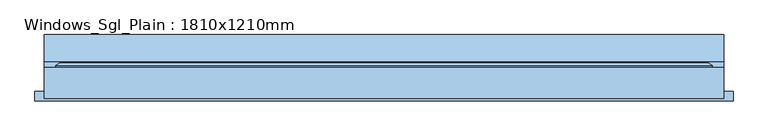
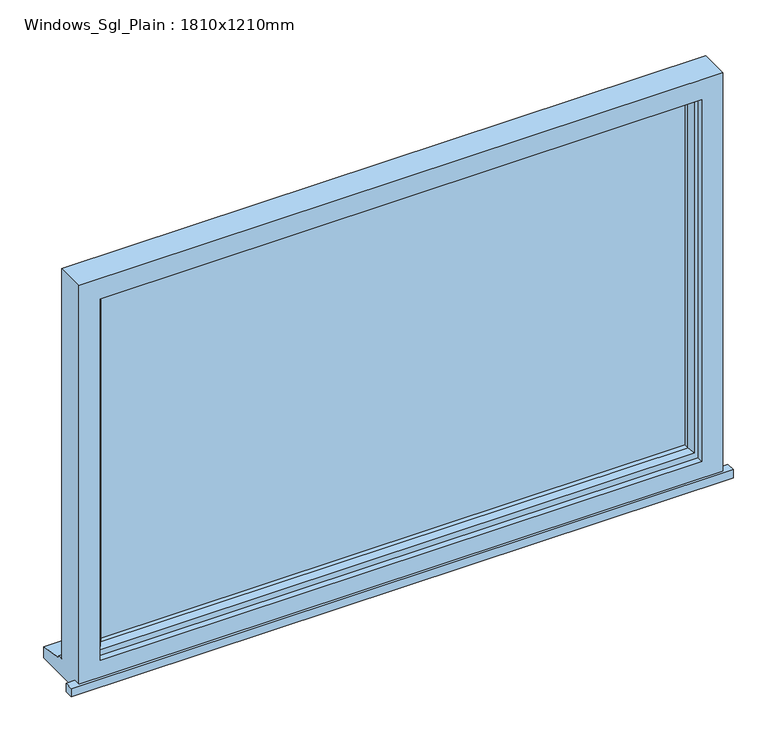
"""IFC4 building model written with IfcOpenShell, lengths in millimetres: window geometry, Windows_Sgl_Plain : 1810x1210mm."""

from ifc_helpers import new_model, si_unit, frame, origin, place, context, project, spatial, polyline, outline, extrude, faceted_brep, source, transform, mapped, element, save


def windows_sgl_plain_1810x1210mm_100c968f(model_context):
    return source(origin(), model_context, "Body", "SolidModel", [
        extrude(outline(polyline([(-930.0, -73.6934322), (-930.0, -48.6934322), (-905.0, -48.6934322), (-905.0, -67.3934322), (905.0, -67.3934322), (905.0, -48.6934322), (930.0, -48.6934322), (930.0, -73.6934322), (-930.0, -73.6934322)])), frame((0.0, 0.0, 900.0), z_axis=(0.0, 0.0, 1.0), x_axis=(1.0, 0.0, 0.0)), (0.0, 0.0, 1.0), 25.0),
        faceted_brep([(-905.0, -67.3934322, 900.0), (905.0, -67.3934322, 900.0), (905.0, -67.3934322, 2110.0), (-905.0, -67.3934322, 2110.0), (-845.0, -67.3934322, 2050.0), (845.0, -67.3934322, 2050.0), (845.0, -67.3934322, 975.0), (-845.0, -67.3934322, 975.0), (-905.0, 15.6065678, 2110.0), (-905.0, 15.6065678, 951.0), (-905.0, 30.6065678, 949.68767), (-905.0, 30.6065678, 944.7449676), (-905.0, 103.1065678, 933.8088847), (-905.0, 103.1065678, 900.0), (905.0, 15.6065678, 2110.0), (905.0, 15.6065678, 951.0), (-865.0, 15.6065678, 2070.0), (-865.0, 15.6065678, 963.0), (865.0, 15.6065678, 963.0), (865.0, 15.6065678, 2070.0), (-865.0, -49.3934322, 2070.0), (-865.0, -49.3934322, 963.0), (865.0, -49.3934322, 2070.0), (865.0, -49.3934322, 963.0), (-845.0, -49.3934322, 2050.0), (-845.0, -49.3934322, 975.0), (845.0, -49.3934322, 975.0), (845.0, -49.3934322, 2050.0), (905.0, 103.1065678, 900.0), (905.0, 103.1065678, 933.8088847), (905.0, 30.6065678, 944.7449676), (905.0, 30.6065678, 949.68767)], [[[0, 1, 2, 3], [4, 5, 6, 7]], [[0, 3, 8, 9, 10, 11, 12, 13]], [[9, 8, 14, 15], [16, 17, 18, 19]], [[17, 16, 20, 21]], [[20, 22, 23, 21], [24, 25, 26, 27]], [[24, 4, 7, 25]], [[3, 2, 14, 8]], [[16, 19, 22, 20]], [[5, 4, 24, 27]], [[15, 14, 2, 1, 28, 29, 30, 31]], [[19, 18, 23, 22]], [[5, 27, 26, 6]], [[28, 1, 0, 13]], [[29, 28, 13, 12]], [[30, 29, 12, 11]], [[31, 30, 11, 10]], [[15, 31, 10, 9]], [[21, 23, 18, 17]], [[7, 6, 26, 25]]]),
        extrude(outline(polyline([(835.0, -20.3934322), (-835.0, -20.3934322), (-835.0, 3.6065678), (835.0, 3.6065678), (835.0, -20.3934322)])), frame((0.0, 0.0, 993.0), z_axis=(0.0, 0.0, 1.0), x_axis=(1.0, 0.0, 0.0)), (0.0, 0.0, 1.0), 1047.0),
        faceted_brep([(-875.0, 15.6065678, 2080.0), (-875.0, 21.3800705, 2080.0), (-875.0, 21.3800705, 953.0), (-875.0, 15.6065678, 953.0), (-865.0, -49.3934322, 2070.0), (-865.0, 15.6065678, 2070.0), (-865.0, 15.6065678, 963.0), (-865.0, -49.3934322, 963.0), (-825.0, -34.9005323, 2030.0), (-835.1480377, -49.3934322, 2040.1480377), (-835.1480377, -49.3934322, 992.8519623), (-825.0, -34.9005323, 1003.0), (-825.0, -20.3934322, 2030.0), (-825.0, -20.3934322, 1003.0), (-835.0, 3.6065678, 2040.0), (-835.0, -20.3934322, 2040.0), (-835.0, -20.3934322, 993.0), (-835.0, 3.6065678, 993.0), (-825.0, 21.3800705, 2030.0), (-825.0, 3.6065678, 2030.0), (-825.0, 3.6065678, 1003.0), (-825.0, 21.3800705, 1003.0), (-842.4457548, 27.1535732, 2047.4457548), (-842.4457548, 27.1535732, 985.5542452), (-864.2153903, 27.1535732, 2069.2153903), (-864.2153903, 27.1535732, 963.7846097), (875.0, 21.3800705, 953.0), (875.0, 15.6065678, 953.0), (865.0, 15.6065678, 963.0), (865.0, -49.3934322, 963.0), (835.1480377, -49.3934322, 992.8519623), (825.0, -34.9005323, 1003.0), (825.0, -20.3934322, 1003.0), (835.0, -20.3934322, 993.0), (835.0, 3.6065678, 993.0), (825.0, 3.6065678, 1003.0), (825.0, 21.3800705, 1003.0), (842.4457548, 27.1535732, 985.5542452), (864.2153903, 27.1535732, 963.7846097), (875.0, 21.3800705, 2080.0), (875.0, 15.6065678, 2080.0), (865.0, 15.6065678, 2070.0), (865.0, -49.3934322, 2070.0), (835.1480377, -49.3934322, 2040.1480377), (825.0, -34.9005323, 2030.0), (825.0, -20.3934322, 2030.0), (835.0, -20.3934322, 2040.0), (835.0, 3.6065678, 2040.0), (825.0, 3.6065678, 2030.0), (825.0, 21.3800705, 2030.0), (842.4457548, 27.1535732, 2047.4457548), (864.2153903, 27.1535732, 2069.2153903)], [[[0, 1, 2, 3]], [[4, 5, 6, 7]], [[8, 9, 10, 11]], [[12, 8, 11, 13]], [[14, 15, 16, 17]], [[18, 19, 20, 21]], [[22, 18, 21, 23]], [[1, 24, 25, 2]], [[3, 2, 26, 27]], [[7, 6, 28, 29]], [[11, 10, 30, 31]], [[13, 11, 31, 32]], [[17, 16, 33, 34]], [[21, 20, 35, 36]], [[23, 21, 36, 37]], [[2, 25, 38, 26]], [[27, 26, 39, 40]], [[29, 28, 41, 42]], [[31, 30, 43, 44]], [[32, 31, 44, 45]], [[34, 33, 46, 47]], [[36, 35, 48, 49]], [[37, 36, 49, 50]], [[26, 38, 51, 39]], [[40, 39, 1, 0]], [[3, 27, 40, 0], [5, 41, 28, 6]], [[42, 41, 5, 4]], [[7, 29, 42, 4], [9, 43, 30, 10]], [[44, 43, 9, 8]], [[45, 44, 8, 12]], [[15, 46, 33, 16], [13, 32, 45, 12]], [[47, 46, 15, 14]], [[17, 34, 47, 14], [19, 48, 35, 20]], [[49, 48, 19, 18]], [[50, 49, 18, 22]], [[24, 51, 38, 25], [23, 37, 50, 22]], [[39, 51, 24, 1]]]),
    ])


if __name__ == "__main__":
    model = new_model("IFC4")
    model_context = context("Model", 3, world=origin())
    ifc_project = project(units=[si_unit("LENGTHUNIT", "METRE", prefix="MILLI")], contexts=[model_context])
    site = spatial("IfcSite", under=ifc_project)
    building = spatial("IfcBuilding", under=site)
    placement = place(None, origin())
    windows_sgl_plain_1810x1210mm_shape = windows_sgl_plain_1810x1210mm_100c968f(model_context)
    element("IfcWindow", 1, ObjectType="Windows_Sgl_Plain : 1810x1210mm", at=placement, inside=building, context=model_context, shape_type="MappedRepresentation", body=[
        mapped(windows_sgl_plain_1810x1210mm_shape, transform((0.0, 0.0, 0.0), x_axis=(1.0, 0.0, 0.0), y_axis=(0.0, 1.0, 0.0), z_axis=(0.0, 0.0, 1.0))),
    ])
    save(model, "model.ifc")

# Revit data of these elements
# Type "Windows_Sgl_Plain : 1810x1210mm"
#   Type Mark = "49"
#   Operation = "SinglePanel"
#   Construction Type Id = "SGL"
#   Manufacturer = "Revit"
#   Keynote = "L10"
#   Analytic Construction = "Large single-glazed windows"
#   Wrap Layers (Ext) from Ext = 102.5 mm
#   Wrap Layers (Int) from Ext = 177.5 mm
#   Window Board Projection = 25 mm
#   Window Board Extension = 25 mm
#   Visual Light Transmittance = 0.9
#   Solar Heat Gain Coefficient = 0.86
#   Rough Width = 1810 mm
#   Rough Height = 1210 mm
#   Height = 1210 mm
#   Width = 1810 mm
#   Heat Transfer Coefficient (U) = 5.5617 W/(m²·K)
#   Glazing Thickness = 24 mm
#   FrameOffset - External = 50 mm
#   Frame Depth = 65 mm
#   Default Head Height = 2110 mm
#   Cill Depth = 87.5 mm
#   Cavity Closer Width = 50 mm
#   Cavity Closer Offset from Ext = 102.5 mm
#   Cavity Closer Depth = 85 mm
#   Define Thermal Properties by = 1
#   Vis - Cavity Closers = yes
#   Define Thermal Properties by = 1
#   Material Trim = Window Frame
#   Material Glass = Glass
#   Material Frame = Window Frame
#   Wall Closure = (empty or 0)
# Element 1 (IfcWindow, "Windows_Sgl_Plain : 1810x1210mm")
#   Materials on its faces: "Window Frame", "Glass"
# Materials
#   "Window Frame": colour RGB 249 249 249, transparency 0, Keynote = "L10", Cost = 0
#   "Glass": class "Glass", colour RGB 0 128 192, transparency 0.9, Description = "Soda Lime Glass", Cost = 0
